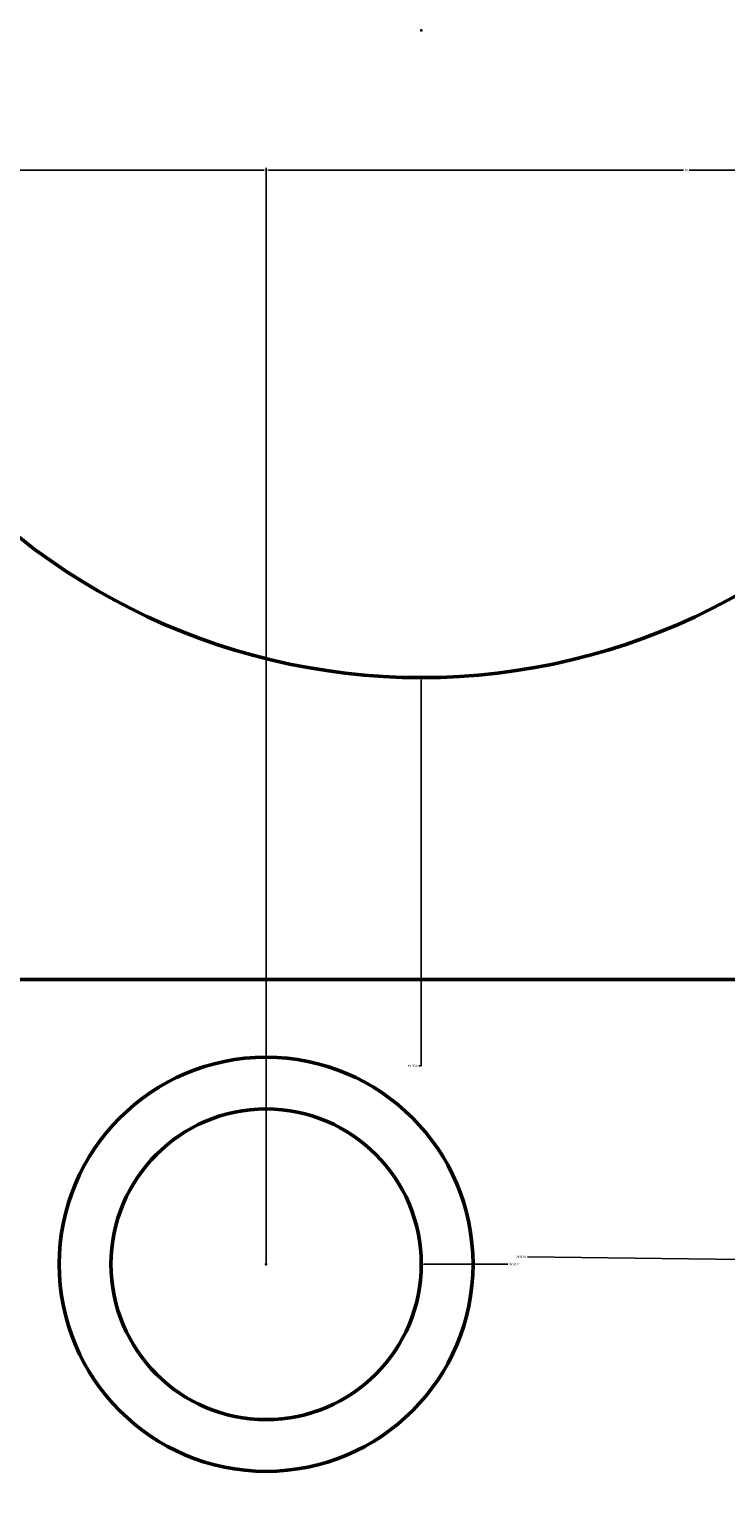
# Model space of a CAD drawing. Units: inches. Extents: x -307 to -76, y 16 to 196.
# Tile 5 of 7: x -222 to -168, y 83 to 196. Entities that reach past the tile are written whole.
import ezdxf

# ---------------------------------------------------------------- set-up
doc = ezdxf.new("R2010")
doc.units = ezdxf.units.IN
doc.header["$MEASUREMENT"] = 0
doc.layers.add('M-DIMS', color=2, linetype='Continuous', lineweight=18)
doc.layers.add('M-OUTL', color=7, linetype='Continuous', lineweight=50)
doc.styles.get("Standard").update_dxf_attribs({"font": 'arial.ttf'})
doc.dimstyles.get("Standard").update_dxf_attribs({"dimtxt": 0.18, "dimasz": 0.18, "dimexe": 0.18, "dimexo": 0.0625, "dimgap": 0.09, "dimtad": 0, "dimtih": 1, "dimtoh": 1, "dimdec": 4, "dimzin": 0, "dimdsep": 46, "dimtxsty": 'Standard', "dimcen": 0.09, "dimadec": 0, "dimazin": 0, "dimtfac": 1, "dimtdec": 4, "dimtofl": 0, "dimtmove": 0, "dimatfit": 3, "dimfxl": 1, "dimtolj": 1, "dimtzin": 0, "dimarcsym": 0})

# ---------------------------------------------------------------- blocks, each defined once
blk = doc.blocks.new('BORE-D24-RIM-D32')
for radius in [16, 12]:
    blk.add_circle((16, 16), radius)
blk = doc.blocks.new('*D2')
at = {"layer": 'Defpoints', "color": 0, "transparency": 16777216}
for p in [(-294.39, 101), (-88.39, 101), (-88.39, 16.45)]:
    blk.add_point(p, dxfattribs=at)
at = {"layer": 'M-DIMS', "color": 0, "lineweight": -2, "transparency": 16777216}
for p, q in [((-294.39, 100.94), (-294.39, 16.27)), ((-88.39, 100.94), (-88.39, 16.27)), ((-294.21, 16.45), (-191.68, 16.45)), ((-88.57, 16.45), (-191.1, 16.45))]:
    blk.add_line(p, q, dxfattribs=at)
at = {"layer": 'M-DIMS', "color": 0, "transparency": 16777216}
for points in [[(-294.21, 16.48), (-294.21, 16.42), (-294.39, 16.45)], [(-88.57, 16.48), (-88.57, 16.42), (-88.39, 16.45)]]:
    blk.add_solid(points, dxfattribs=at)
at = {"layer": 'M-DIMS', "color": 0, "transparency": 16777216, "insert": (-191.39, 16.45), "char_height": 0.18, "attachment_point": 5}
blk.add_mtext('\\A1;206', dxfattribs=at)
blk = doc.blocks.new('*D4')
at = {"layer": 'Defpoints', "color": 0, "transparency": 16777216}
for p in [(-203.39, 185.55), (-244.39, 157), (-203.39, 101)]:
    blk.add_point(p, dxfattribs=at)
at = {"layer": 'M-DIMS', "color": 0, "lineweight": -2, "transparency": 16777216}
for p, q in [((-244.39, 157.06), (-244.39, 185.73)), ((-203.39, 101.06), (-203.39, 185.73)), ((-244.21, 185.55), (-224.09, 185.55)), ((-203.57, 185.55), (-223.68, 185.55))]:
    blk.add_line(p, q, dxfattribs=at)
at = {"layer": 'M-DIMS', "color": 0, "transparency": 16777216}
for points in [[(-244.21, 185.58), (-244.21, 185.52), (-244.39, 185.55)], [(-203.57, 185.58), (-203.57, 185.52), (-203.39, 185.55)]]:
    blk.add_solid(points, dxfattribs=at)
at = {"layer": 'M-DIMS', "color": 0, "transparency": 16777216, "insert": (-223.89, 185.55), "char_height": 0.18, "attachment_point": 5}
blk.add_mtext('\\A1;41', dxfattribs=at)
blk = doc.blocks.new('*D5')
at = {"layer": 'Defpoints', "color": 0, "transparency": 16777216}
for p in [(-138.39, 185.55), (-138.39, 157), (-203.39, 101)]:
    blk.add_point(p, dxfattribs=at)
at = {"layer": 'M-DIMS', "color": 0, "lineweight": -2, "transparency": 16777216}
for p, q in [((-203.39, 101.06), (-203.39, 185.73)), ((-138.39, 157.06), (-138.39, 185.73)), ((-203.21, 185.55), (-171.11, 185.55)), ((-138.57, 185.55), (-170.67, 185.55))]:
    blk.add_line(p, q, dxfattribs=at)
at = {"layer": 'M-DIMS', "color": 0, "transparency": 16777216}
for points in [[(-203.21, 185.58), (-203.21, 185.52), (-203.39, 185.55)], [(-138.57, 185.58), (-138.57, 185.52), (-138.39, 185.55)]]:
    blk.add_solid(points, dxfattribs=at)
at = {"layer": 'M-DIMS', "color": 0, "transparency": 16777216, "insert": (-170.89, 185.55), "char_height": 0.18, "attachment_point": 5}
blk.add_mtext('\\A1;65', dxfattribs=at)
blk = doc.blocks.new('*D10')
at = {"layer": 'Defpoints', "color": 0, "transparency": 16777216}
for p in [(-191.39, 196.33), (-191.39, 146.33)]:
    blk.add_point(p, dxfattribs=at)
at = {"layer": 'M-DIMS', "color": 0, "lineweight": -2, "transparency": 16777216}
for p, q in [((-191.48, 196.33), (-191.3, 196.33)), ((-191.39, 196.24), (-191.39, 196.42)), ((-191.39, 116.33), (-191.39, 146.15)), ((-191.57, 116.33), (-191.39, 116.33))]:
    blk.add_line(p, q, dxfattribs=at)
at = {"layer": 'M-DIMS', "color": 0, "transparency": 16777216}
blk.add_solid([(-191.42, 146.15), (-191.36, 146.15), (-191.39, 146.33)], dxfattribs=at)
at = {"layer": 'M-DIMS', "color": 0, "transparency": 16777216, "insert": (-192.07, 116.33), "char_height": 0.18, "attachment_point": 5}
blk.add_mtext('\\A1;4X R50', dxfattribs=at)
blk = doc.blocks.new('*D14')
at = {"layer": 'Defpoints', "color": 0, "transparency": 16777216}
for p in [(-166.39, 101.35), (-138.39, 101)]:
    blk.add_point(p, dxfattribs=at)
at = {"layer": 'M-DIMS', "color": 0, "lineweight": -2, "transparency": 16777216}
for p, q in [((-183.19, 101.57), (-166.57, 101.36)), ((-138.48, 101), (-138.3, 101)), ((-138.39, 100.91), (-138.39, 101.09))]:
    blk.add_line(p, q, dxfattribs=at)
at = {"layer": 'M-DIMS', "color": 0, "transparency": 16777216}
blk.add_solid([(-166.57, 101.39), (-166.57, 101.33), (-166.39, 101.35)], dxfattribs=at)
at = {"layer": 'M-DIMS', "color": 0, "transparency": 16777216, "insert": (-183.69, 101.57), "char_height": 0.18, "attachment_point": 5}
blk.add_mtext('\\A1;2X R28', dxfattribs=at)
blk = doc.blocks.new('*D19')
at = {"layer": 'Defpoints', "color": 0, "transparency": 16777216}
for p in [(-215.39, 101), (-191.39, 101)]:
    blk.add_point(p, dxfattribs=at)
at = {"layer": 'M-DIMS', "color": 0, "lineweight": -2, "transparency": 16777216}
for p, q in [((-203.48, 101), (-203.3, 101)), ((-203.39, 100.91), (-203.39, 101.09)), ((-184.7, 101), (-191.21, 101))]:
    blk.add_line(p, q, dxfattribs=at)
at = {"layer": 'M-DIMS', "color": 0, "transparency": 16777216}
blk.add_solid([(-191.21, 101.03), (-191.21, 100.97), (-191.39, 101)], dxfattribs=at)
at = {"layer": 'M-DIMS', "color": 0, "transparency": 16777216, "insert": (-184.19, 101), "char_height": 0.18, "attachment_point": 5}
blk.add_mtext('\\A1;4X ∅24', dxfattribs=at)

msp = doc.modelspace()

# ---------------------------------------------------------------- linework, layer by layer
at = {"layer": 'M-OUTL'}
msp.add_line((-244.39, 123), (-159.19, 123), dxfattribs=at)
msp.add_arc((-191.39, 196.33), 50, 216.5795, 323.4205, dxfattribs=at)

# ---------------------------------------------------------------- block references
msp.add_blockref('BORE-D24-RIM-D32', (-219.39, 85), dxfattribs=at)

# ---------------------------------------------------------------- dimensions: what is measured, and where the dimension line sits
at = {"layer": 'M-DIMS'}
for center, mpoint, text, picture, middle in [((-191.39, 196.33), (-191.39, 146.33), '4X <>', '*D10', (-192.07, 116.33)), ((-138.39, 101), (-166.39, 101.35), '2X <>', '*D14', (-183.19, 101.57))]:
    dim = msp.add_radius_dim(center=center, mpoint=mpoint, text=text, dimstyle='Standard', override={"dimdec": 0, "dimlfac": 1, "dimrnd": 0, "dimzin": 0, "dimdsep": 46, "dimlunit": 2}, dxfattribs=at)
    dim.commit()
    dim.dimension.update_dxf_attribs({"geometry": picture, "text_midpoint": middle, "dimtype": 164})
for base, p1, p2, picture, middle in [((-203.39, 185.55), (-244.39, 157), (-203.39, 101), '*D4', (-223.89, 185.55)), ((-138.39, 185.55), (-203.39, 101), (-138.39, 157), '*D5', (-170.89, 185.55)), ((-88.39, 16.45), (-294.39, 101), (-88.39, 101), '*D2', (-191.39, 16.45))]:
    dim = msp.add_linear_dim(base=base, p1=p1, p2=p2, dimstyle='Standard', override={"dimdec": 0, "dimlfac": 1, "dimrnd": 0, "dimzin": 0, "dimdsep": 46, "dimlunit": 2}, dxfattribs=at)
    dim.commit()
    dim.dimension.update_dxf_attribs({"geometry": picture, "text_midpoint": middle})
dim = msp.add_diameter_dim_2p(p1=(-215.39, 101), p2=(-191.39, 101), text='4X <>', dimstyle='Standard', override={"dimdec": 0, "dimlfac": 1, "dimrnd": 0, "dimzin": 0, "dimdsep": 46, "dimlunit": 2}, dxfattribs=at)
dim.commit()
dim.dimension.update_dxf_attribs({"geometry": '*D19', "text_midpoint": (-184.19, 101), "dimtype": 163})

doc.saveas('drawing.dxf')
